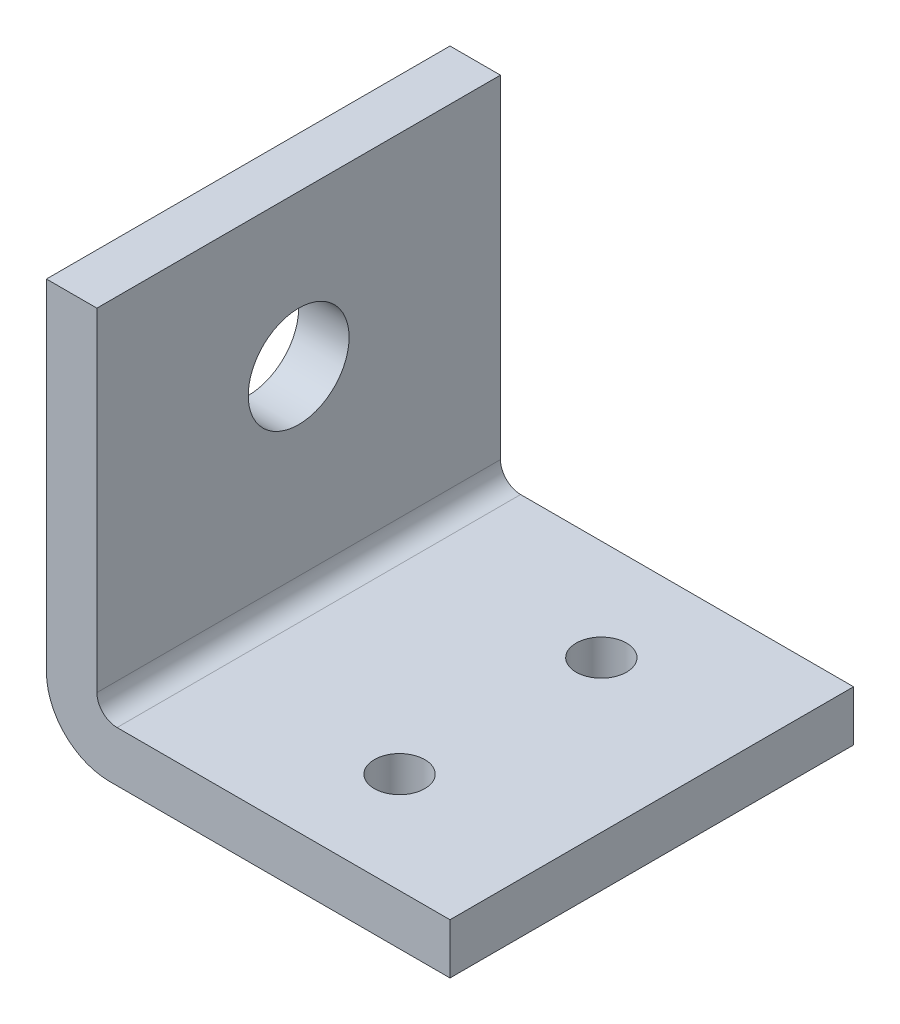
SolidWorks part; units mm, degrees
material "Plain Carbon Steel"
ref_plane "Front Plane" through (0, 0, 0) normal (0, 0, 1) x (1, 0, 0)
ref_plane "Top Plane" through (0, 0, 0) normal (0, 1, 0) x (1, 0, 0)
ref_plane "Right Plane" through (0, 0, 0) normal (1, 0, 0) x (0, 0, -1)
sketch "Bracket Profile Sketch" plane through (0, 0, 0) normal (0, 0, 1) x (1, 0, 0)
  line L0 (0, 6.25) -> (0, 40)
  line L1 (6.25, 0) -> (40, 0)
  line L2 (5, 7) -> (5, 40)
  line L3 (7, 5) -> (40, 5)
  line L4 (40, 0) -> (40, 5)
  line L5 (0, 40) -> (5, 40)
  line L6 (0, 0) -> (40, 0) construction
  line L7 (0, 0) -> (0, 40) construction
  line L8 (5, 5) -> (40, 5) construction
  line L9 (5, 5) -> (5, 40) construction
  arc A0 (6.25, 0) -> (0, 6.25) centre (6.25, 6.25) cw
  arc A1 (7, 5) -> (5, 7) centre (7, 7) cw
  point P10 (0, 0)
  dimension "D4" = 6.25
  dimension "D5" = 2
  dimension "D1" = 40
  dimension "D2" = 40
  dimension "D3" = 5
extrude "L-Bracket Body" add sketch "Bracket Profile Sketch" along normal mid plane 40
sketch "Upright Hole Sketch" plane through (5, 0, 0) normal (1, 0, 0) x (0, 0, -1)
  circle A0 centre (0, 25) radius 5
  dimension "D1" = 10
  dimension "D4" = 25
extrude "Upright Hole Ø10" cut sketch "Upright Hole Sketch" against normal through all
sketch "Base Holes Sketch" plane through (0, 5, 0) normal (0, 1, 0) x (1, 0, 0)
  circle A0 centre (25, 10) radius 2.5
  circle A1 centre (25, -10) radius 2.5
  dimension "D1" = 5
  dimension "D2" = 10
  dimension "D3" = 20
  dimension "15" = 15
extrude "Base Holes 2xØ5" cut sketch "Base Holes Sketch" against normal through all
